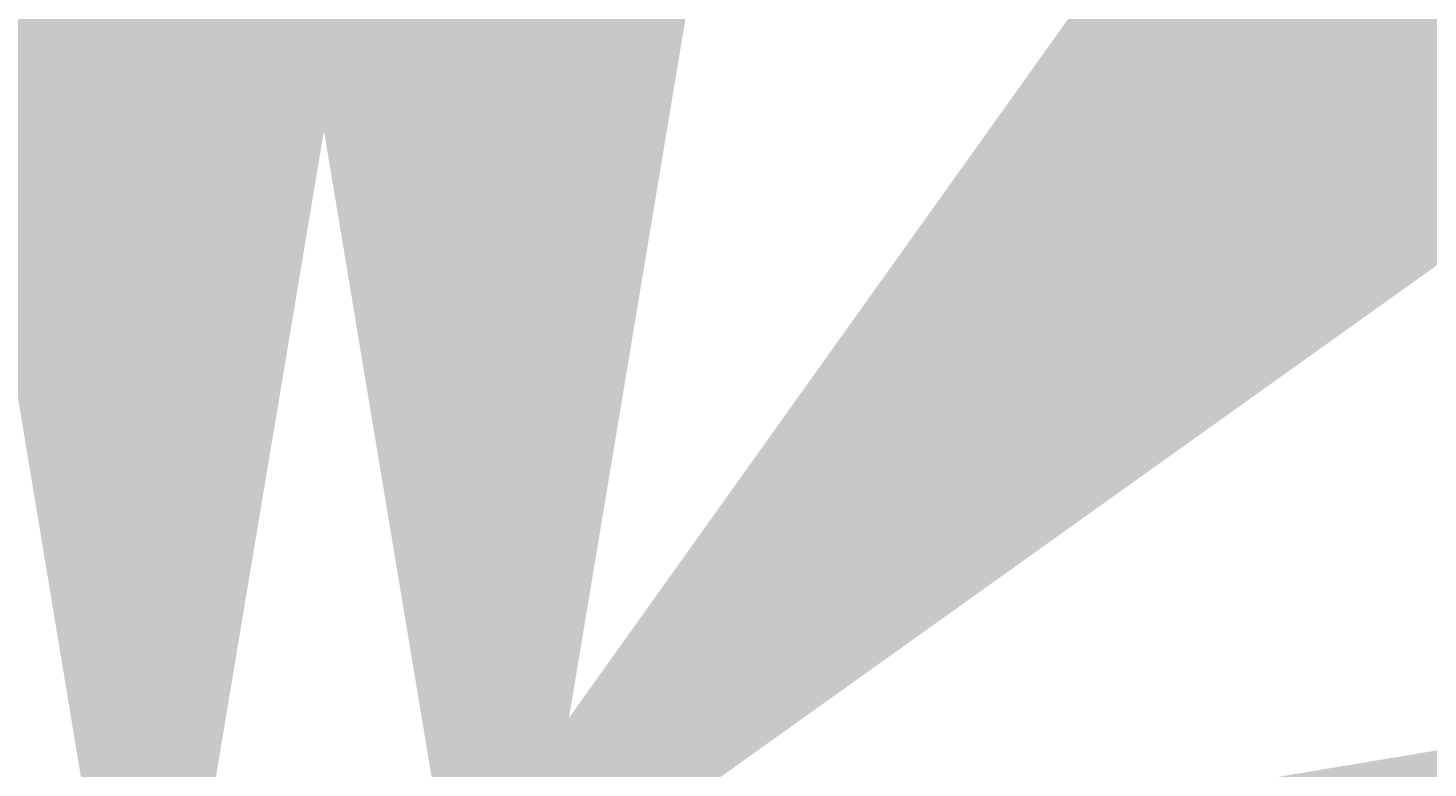
# Model space of a CAD drawing. Units: millimetres. Extents: x -22994 to 29398, y -19990 to 20176.
# Tile 128 of 135: x -44 to 1004, y 341 to 895. Entities that reach past the tile are written whole.
import ezdxf

# ---------------------------------------------------------------- set-up
doc = ezdxf.new("R2010")
doc.units = ezdxf.units.MM
doc.header["$MEASUREMENT"] = 0
doc.layers.add('M-DIMS', color=2, linetype='Continuous', lineweight=18)
doc.styles.get("Standard").update_dxf_attribs({"font": 'arial.ttf'})
doc.dimstyles.get("Standard").update_dxf_attribs({"dimtxt": 0.18, "dimasz": 10000, "dimexe": 0.18, "dimexo": 0.0625, "dimgap": 0.09, "dimtad": 0, "dimtih": 1, "dimtoh": 1, "dimdec": 0, "dimzin": 0, "dimdsep": 46, "dimtxsty": 'Standard', "dimcen": 0.09, "dimadec": 0, "dimazin": 0, "dimtfac": 1, "dimtdec": 0, "dimtofl": 0, "dimtmove": 0, "dimatfit": 3, "dimfxl": 1, "dimtolj": 1, "dimtzin": 0, "dimlwd": 30, "dimarcsym": 0})

# ---------------------------------------------------------------- blocks, each defined once
blk = doc.blocks.new('*D2')
at = {"layer": 'Defpoints', "color": 0, "transparency": 16777216}
for p in [(6.7, 10.3), (290.9, 10.3), (290.9, -5.1)]:
    blk.add_point(p, dxfattribs=at)
at = {"layer": 'M-DIMS', "color": 0, "lineweight": -2, "transparency": 16777216}
for p, q in [((6.7, 10.2), (6.7, -5.3)), ((290.9, 10.2), (290.9, -5.3))]:
    blk.add_line(p, q, dxfattribs=at)
at = {"layer": 'M-DIMS', "color": 0, "lineweight": 30, "transparency": 16777216}
for p, q in [((-9993.3, -5.1), (-19993.3, -5.1)), ((10290.9, -5.1), (20290.9, -5.1))]:
    blk.add_line(p, q, dxfattribs=at)
at = {"layer": 'M-DIMS', "color": 0, "transparency": 16777216}
for points in [[(-9993.3, 1661.6), (-9993.3, -1671.7), (6.7, -5.1)], [(10290.9, 1661.6), (10290.9, -1671.7), (290.9, -5.1)]]:
    blk.add_solid(points, dxfattribs=at)
at = {"layer": 'M-DIMS', "color": 0, "transparency": 16777216, "insert": (148.8, -5.1), "char_height": 0.18, "attachment_point": 5}
blk.add_mtext('\\A1;284.2', dxfattribs=at)
blk = doc.blocks.new('*D3')
at = {"layer": 'Defpoints', "color": 0, "transparency": 16777216}
for p in [(110.3, 204.2), (110.3, 176.4), (95.8, 128)]:
    blk.add_point(p, dxfattribs=at)
at = {"layer": 'M-DIMS', "color": 0, "lineweight": 30, "transparency": 16777216}
for p, q in [((-9904.2, 204.2), (-19904.2, 204.2)), ((10110.3, 204.2), (20110.3, 204.2))]:
    blk.add_line(p, q, dxfattribs=at)
at = {"layer": 'M-DIMS', "color": 0, "lineweight": -2, "transparency": 16777216}
for p, q in [((95.8, 128), (95.8, 204.3)), ((110.3, 176.4), (110.3, 204.3))]:
    blk.add_line(p, q, dxfattribs=at)
at = {"layer": 'M-DIMS', "color": 0, "transparency": 16777216}
for points in [[(-9904.2, 1870.8), (-9904.2, -1462.5), (95.8, 204.2)], [(10110.3, 1870.8), (10110.3, -1462.5), (110.3, 204.2)]]:
    blk.add_solid(points, dxfattribs=at)
at = {"layer": 'M-DIMS', "color": 0, "transparency": 16777216, "insert": (103, 204.2), "char_height": 0.18, "attachment_point": 5}
blk.add_mtext('\\A1;14.432', dxfattribs=at)
blk = doc.blocks.new('*D4')
at = {"layer": 'Defpoints', "color": 0, "transparency": 16777216}
for p in [(116.3, 204.2), (110.3, 176.4), (116.3, 176.4)]:
    blk.add_point(p, dxfattribs=at)
at = {"layer": 'M-DIMS', "color": 0, "lineweight": 30, "transparency": 16777216}
for p, q in [((-9889.7, 204.2), (-19889.7, 204.2)), ((10116.3, 204.2), (20116.3, 204.2))]:
    blk.add_line(p, q, dxfattribs=at)
at = {"layer": 'M-DIMS', "color": 0, "lineweight": -2, "transparency": 16777216}
for p, q in [((110.3, 176.4), (110.3, 204.3)), ((116.3, 176.4), (116.3, 204.3))]:
    blk.add_line(p, q, dxfattribs=at)
at = {"layer": 'M-DIMS', "color": 0, "transparency": 16777216}
for points in [[(-9889.7, 1870.8), (-9889.7, -1462.5), (110.3, 204.2)], [(10116.3, 1870.8), (10116.3, -1462.5), (116.3, 204.2)]]:
    blk.add_solid(points, dxfattribs=at)
at = {"layer": 'M-DIMS', "color": 0, "transparency": 16777216, "insert": (113.3, 204.2), "char_height": 0.18, "attachment_point": 5}
blk.add_mtext('\\A1;6', dxfattribs=at)
blk = doc.blocks.new('*D5')
at = {"layer": 'Defpoints', "color": 0, "transparency": 16777216}
for p in [(181.3, 204.2), (116.3, 176.4), (181.3, 176.4)]:
    blk.add_point(p, dxfattribs=at)
at = {"layer": 'M-DIMS', "color": 0, "lineweight": 30, "transparency": 16777216}
for p, q in [((-9883.7, 204.2), (-19883.7, 204.2)), ((10181.3, 204.2), (20181.3, 204.2))]:
    blk.add_line(p, q, dxfattribs=at)
at = {"layer": 'M-DIMS', "color": 0, "lineweight": -2, "transparency": 16777216}
for p, q in [((116.3, 176.4), (116.3, 204.3)), ((181.3, 176.4), (181.3, 204.3))]:
    blk.add_line(p, q, dxfattribs=at)
at = {"layer": 'M-DIMS', "color": 0, "transparency": 16777216}
for points in [[(-9883.7, 1870.8), (-9883.7, -1462.5), (116.3, 204.2)], [(10181.3, 1870.8), (10181.3, -1462.5), (181.3, 204.2)]]:
    blk.add_solid(points, dxfattribs=at)
at = {"layer": 'M-DIMS', "color": 0, "transparency": 16777216, "insert": (148.8, 204.2), "char_height": 0.18, "attachment_point": 5}
blk.add_mtext('\\A1;65', dxfattribs=at)
blk = doc.blocks.new('*D6')
at = {"layer": 'Defpoints', "color": 0, "transparency": 16777216}
for p in [(187.3, 204.2), (181.3, 176.4), (187.3, 176.4)]:
    blk.add_point(p, dxfattribs=at)
at = {"layer": 'M-DIMS', "color": 0, "lineweight": 30, "transparency": 16777216}
for p, q in [((-9818.7, 204.2), (-19818.7, 204.2)), ((10187.3, 204.2), (20187.3, 204.2))]:
    blk.add_line(p, q, dxfattribs=at)
at = {"layer": 'M-DIMS', "color": 0, "lineweight": -2, "transparency": 16777216}
for p, q in [((181.3, 176.4), (181.3, 204.3)), ((187.3, 176.4), (187.3, 204.3))]:
    blk.add_line(p, q, dxfattribs=at)
at = {"layer": 'M-DIMS', "color": 0, "transparency": 16777216}
for points in [[(-9818.7, 1870.8), (-9818.7, -1462.5), (181.3, 204.2)], [(10187.3, 1870.8), (10187.3, -1462.5), (187.3, 204.2)]]:
    blk.add_solid(points, dxfattribs=at)
at = {"layer": 'M-DIMS', "color": 0, "transparency": 16777216, "insert": (184.3, 204.2), "char_height": 0.18, "attachment_point": 5}
blk.add_mtext('\\A1;6', dxfattribs=at)
blk = doc.blocks.new('*D7')
at = {"layer": 'Defpoints', "color": 0, "transparency": 16777216}
for p in [(201.7, 204.2), (187.3, 176.4), (201.7, 128)]:
    blk.add_point(p, dxfattribs=at)
at = {"layer": 'M-DIMS', "color": 0, "lineweight": 30, "transparency": 16777216}
for p, q in [((-9812.7, 204.2), (-19812.7, 204.2)), ((10201.7, 204.2), (20201.7, 204.2))]:
    blk.add_line(p, q, dxfattribs=at)
at = {"layer": 'M-DIMS', "color": 0, "lineweight": -2, "transparency": 16777216}
for p, q in [((187.3, 176.4), (187.3, 204.3)), ((201.7, 128), (201.7, 204.3))]:
    blk.add_line(p, q, dxfattribs=at)
at = {"layer": 'M-DIMS', "color": 0, "transparency": 16777216}
for points in [[(-9812.7, 1870.8), (-9812.7, -1462.5), (187.3, 204.2)], [(10201.7, 1870.8), (10201.7, -1462.5), (201.7, 204.2)]]:
    blk.add_solid(points, dxfattribs=at)
at = {"layer": 'M-DIMS', "color": 0, "transparency": 16777216, "insert": (194.5, 204.2), "char_height": 0.18, "attachment_point": 5}
blk.add_mtext('\\A1;14.432', dxfattribs=at)
blk = doc.blocks.new('*D8')
at = {"layer": 'Defpoints', "color": 0, "transparency": 16777216}
for p in [(227.6, 204.2), (227.6, 146.7), (201.7, 128)]:
    blk.add_point(p, dxfattribs=at)
at = {"layer": 'M-DIMS', "color": 0, "lineweight": 30, "transparency": 16777216}
for p, q in [((-9798.3, 204.2), (-19798.3, 204.2)), ((10227.6, 204.2), (20227.6, 204.2))]:
    blk.add_line(p, q, dxfattribs=at)
at = {"layer": 'M-DIMS', "color": 0, "lineweight": -2, "transparency": 16777216}
for p, q in [((201.7, 128), (201.7, 204.3)), ((227.6, 146.8), (227.6, 204.3))]:
    blk.add_line(p, q, dxfattribs=at)
at = {"layer": 'M-DIMS', "color": 0, "transparency": 16777216}
for points in [[(-9798.3, 1870.8), (-9798.3, -1462.5), (201.7, 204.2)], [(10227.6, 1870.8), (10227.6, -1462.5), (227.6, 204.2)]]:
    blk.add_solid(points, dxfattribs=at)
at = {"layer": 'M-DIMS', "color": 0, "transparency": 16777216, "insert": (214.7, 204.2), "char_height": 0.18, "attachment_point": 5}
blk.add_mtext('\\A1;25.95', dxfattribs=at)
blk = doc.blocks.new('*D9')
at = {"layer": 'Defpoints', "color": 0, "transparency": 16777216}
for p in [(187.3, 176.4), (306.2, 176.4), (290.9, 10.3)]:
    blk.add_point(p, dxfattribs=at)
at = {"layer": 'M-DIMS', "color": 0, "lineweight": 30, "transparency": 16777216}
for p, q in [((306.2, 10176.4), (306.2, 20176.4)), ((306.2, -9989.7), (306.2, -19989.7))]:
    blk.add_line(p, q, dxfattribs=at)
at = {"layer": 'M-DIMS', "color": 0, "lineweight": -2, "transparency": 16777216}
for p, q in [((187.3, 176.4), (306.4, 176.4)), ((290.9, 10.3), (306.4, 10.3))]:
    blk.add_line(p, q, dxfattribs=at)
at = {"layer": 'M-DIMS', "color": 0, "transparency": 16777216}
for points in [[(-1360.5, 10176.4), (1972.9, 10176.4), (306.2, 176.4)], [(-1360.5, -9989.7), (1972.9, -9989.7), (306.2, 10.3)]]:
    blk.add_solid(points, dxfattribs=at)
at = {"layer": 'M-DIMS', "color": 0, "transparency": 16777216, "insert": (306.2, 93.3), "char_height": 0.18, "attachment_point": 5}
blk.add_mtext('\\A1;166.1', dxfattribs=at)
blk = doc.blocks.new('*D10')
at = {"layer": 'Defpoints', "color": 0, "transparency": 16777216}
for p in [(125.6, 136.1), (133.3, 136.1), (133.3, -5.1)]:
    blk.add_point(p, dxfattribs=at)
at = {"layer": 'M-DIMS', "color": 0, "lineweight": -2, "transparency": 16777216}
for p, q in [((125.6, 136), (125.6, -5.3)), ((133.3, 136), (133.3, -5.3))]:
    blk.add_line(p, q, dxfattribs=at)
at = {"layer": 'M-DIMS', "color": 0, "lineweight": 30, "transparency": 16777216}
for p, q in [((-9874.4, -5.1), (-19874.4, -5.1)), ((10133.3, -5.1), (20133.3, -5.1))]:
    blk.add_line(p, q, dxfattribs=at)
at = {"layer": 'M-DIMS', "color": 0, "transparency": 16777216}
for points in [[(-9874.4, 1661.6), (-9874.4, -1671.7), (125.6, -5.1)], [(10133.3, 1661.6), (10133.3, -1671.7), (133.3, -5.1)]]:
    blk.add_solid(points, dxfattribs=at)
at = {"layer": 'M-DIMS', "color": 0, "transparency": 16777216, "insert": (129.5, -5.1), "char_height": 0.18, "attachment_point": 5}
blk.add_mtext('\\A1;7.696', dxfattribs=at)
blk = doc.blocks.new('*D11')
at = {"layer": 'Defpoints', "color": 0, "transparency": 16777216}
for p in [(133.3, 136.1), (135.6, 136.1), (135.6, -5.1)]:
    blk.add_point(p, dxfattribs=at)
at = {"layer": 'M-DIMS', "color": 0, "lineweight": -2, "transparency": 16777216}
for p, q in [((133.3, 136), (133.3, -5.3)), ((135.6, 136), (135.6, -5.3))]:
    blk.add_line(p, q, dxfattribs=at)
at = {"layer": 'M-DIMS', "color": 0, "lineweight": 30, "transparency": 16777216}
for p, q in [((-9866.7, -5.1), (-19866.7, -5.1)), ((10135.6, -5.1), (20135.6, -5.1))]:
    blk.add_line(p, q, dxfattribs=at)
at = {"layer": 'M-DIMS', "color": 0, "transparency": 16777216}
for points in [[(-9866.7, 1661.6), (-9866.7, -1671.7), (133.3, -5.1)], [(10135.6, 1661.6), (10135.6, -1671.7), (135.6, -5.1)]]:
    blk.add_solid(points, dxfattribs=at)
at = {"layer": 'M-DIMS', "color": 0, "transparency": 16777216, "insert": (134.5, -5.1), "char_height": 0.18, "attachment_point": 5}
blk.add_mtext('\\A1;2.304', dxfattribs=at)
blk = doc.blocks.new('*D12')
at = {"layer": 'Defpoints', "color": 0, "transparency": 16777216}
for p in [(135.6, 136.1), (145.6, 136.1), (145.6, -5.1)]:
    blk.add_point(p, dxfattribs=at)
at = {"layer": 'M-DIMS', "color": 0, "lineweight": -2, "transparency": 16777216}
for p, q in [((135.6, 136), (135.6, -5.3)), ((145.6, 136), (145.6, -5.3))]:
    blk.add_line(p, q, dxfattribs=at)
at = {"layer": 'M-DIMS', "color": 0, "lineweight": 30, "transparency": 16777216}
for p, q in [((-9864.4, -5.1), (-19864.4, -5.1)), ((10145.6, -5.1), (20145.6, -5.1))]:
    blk.add_line(p, q, dxfattribs=at)
at = {"layer": 'M-DIMS', "color": 0, "transparency": 16777216}
for points in [[(-9864.4, 1661.6), (-9864.4, -1671.7), (135.6, -5.1)], [(10145.6, 1661.6), (10145.6, -1671.7), (145.6, -5.1)]]:
    blk.add_solid(points, dxfattribs=at)
at = {"layer": 'M-DIMS', "color": 0, "transparency": 16777216, "insert": (140.6, -5.1), "char_height": 0.18, "attachment_point": 5}
blk.add_mtext('\\A1;10', dxfattribs=at)
blk = doc.blocks.new('*D13')
at = {"layer": 'Defpoints', "color": 0, "transparency": 16777216}
for p in [(145.6, 136.1), (155.6, 136.1), (155.6, -5.1)]:
    blk.add_point(p, dxfattribs=at)
at = {"layer": 'M-DIMS', "color": 0, "lineweight": -2, "transparency": 16777216}
for p, q in [((145.6, 136), (145.6, -5.3)), ((155.6, 136), (155.6, -5.3))]:
    blk.add_line(p, q, dxfattribs=at)
at = {"layer": 'M-DIMS', "color": 0, "lineweight": 30, "transparency": 16777216}
for p, q in [((-9854.4, -5.1), (-19854.4, -5.1)), ((10155.6, -5.1), (20155.6, -5.1))]:
    blk.add_line(p, q, dxfattribs=at)
at = {"layer": 'M-DIMS', "color": 0, "transparency": 16777216}
for points in [[(-9854.4, 1661.6), (-9854.4, -1671.7), (145.6, -5.1)], [(10155.6, 1661.6), (10155.6, -1671.7), (155.6, -5.1)]]:
    blk.add_solid(points, dxfattribs=at)
at = {"layer": 'M-DIMS', "color": 0, "transparency": 16777216, "insert": (150.6, -5.1), "char_height": 0.18, "attachment_point": 5}
blk.add_mtext('\\A1;10', dxfattribs=at)
blk = doc.blocks.new('*D14')
at = {"layer": 'Defpoints', "color": 0, "transparency": 16777216}
for p in [(155.6, 136.1), (165.6, 136.1), (165.6, -5.1)]:
    blk.add_point(p, dxfattribs=at)
at = {"layer": 'M-DIMS', "color": 0, "lineweight": -2, "transparency": 16777216}
for p, q in [((155.6, 136), (155.6, -5.3)), ((165.6, 136), (165.6, -5.3))]:
    blk.add_line(p, q, dxfattribs=at)
at = {"layer": 'M-DIMS', "color": 0, "lineweight": 30, "transparency": 16777216}
for p, q in [((-9844.4, -5.1), (-19844.4, -5.1)), ((10165.6, -5.1), (20165.6, -5.1))]:
    blk.add_line(p, q, dxfattribs=at)
at = {"layer": 'M-DIMS', "color": 0, "transparency": 16777216}
for points in [[(-9844.4, 1661.6), (-9844.4, -1671.7), (155.6, -5.1)], [(10165.6, 1661.6), (10165.6, -1671.7), (165.6, -5.1)]]:
    blk.add_solid(points, dxfattribs=at)
at = {"layer": 'M-DIMS', "color": 0, "transparency": 16777216, "insert": (160.6, -5.1), "char_height": 0.18, "attachment_point": 5}
blk.add_mtext('\\A1;10', dxfattribs=at)
blk = doc.blocks.new('*D15')
at = {"layer": 'Defpoints', "color": 0, "transparency": 16777216}
for p in [(173.3, 154.8), (173.3, 136.1), (306.2, 136.1)]:
    blk.add_point(p, dxfattribs=at)
at = {"layer": 'M-DIMS', "color": 0, "lineweight": 30, "transparency": 16777216}
for p, q in [((306.2, 10154.8), (306.2, 20154.8)), ((306.2, -9863.9), (306.2, -19863.9))]:
    blk.add_line(p, q, dxfattribs=at)
at = {"layer": 'M-DIMS', "color": 0, "lineweight": -2, "transparency": 16777216}
for p, q in [((173.4, 154.8), (306.4, 154.8)), ((173.4, 136.1), (306.4, 136.1))]:
    blk.add_line(p, q, dxfattribs=at)
at = {"layer": 'M-DIMS', "color": 0, "transparency": 16777216}
for points in [[(-1360.5, 10154.8), (1972.9, 10154.8), (306.2, 154.8)], [(-1360.5, -9863.9), (1972.9, -9863.9), (306.2, 136.1)]]:
    blk.add_solid(points, dxfattribs=at)
at = {"layer": 'M-DIMS', "color": 0, "transparency": 16777216, "insert": (306.2, 145.4), "char_height": 0.18, "attachment_point": 5}
blk.add_mtext('\\A1;18.717', dxfattribs=at)
blk = doc.blocks.new('*D16')
at = {"layer": 'Defpoints', "color": 0, "transparency": 16777216}
for p in [(120.2, 204.2), (110.5, 48), (120.2, 48)]:
    blk.add_point(p, dxfattribs=at)
at = {"layer": 'M-DIMS', "color": 0, "lineweight": 30, "transparency": 16777216}
for p, q in [((-9889.5, 204.2), (-19889.5, 204.2)), ((10120.2, 204.2), (20120.2, 204.2))]:
    blk.add_line(p, q, dxfattribs=at)
at = {"layer": 'M-DIMS', "color": 0, "lineweight": -2, "transparency": 16777216}
for p, q in [((110.5, 48.1), (110.5, 204.3)), ((120.2, 48.1), (120.2, 204.3))]:
    blk.add_line(p, q, dxfattribs=at)
at = {"layer": 'M-DIMS', "color": 0, "transparency": 16777216}
for points in [[(-9889.5, 1870.8), (-9889.5, -1462.5), (110.5, 204.2)], [(10120.2, 1870.8), (10120.2, -1462.5), (120.2, 204.2)]]:
    blk.add_solid(points, dxfattribs=at)
at = {"layer": 'M-DIMS', "color": 0, "transparency": 16777216, "insert": (115.3, 204.2), "char_height": 0.18, "attachment_point": 5}
blk.add_mtext('\\A1;9.704', dxfattribs=at)
blk = doc.blocks.new('*D17')
at = {"layer": 'Defpoints', "color": 0, "transparency": 16777216}
for p in [(126.2, 204.2), (120.2, 48), (126.2, 48)]:
    blk.add_point(p, dxfattribs=at)
at = {"layer": 'M-DIMS', "color": 0, "lineweight": 30, "transparency": 16777216}
for p, q in [((-9879.8, 204.2), (-19879.8, 204.2)), ((10126.2, 204.2), (20126.2, 204.2))]:
    blk.add_line(p, q, dxfattribs=at)
at = {"layer": 'M-DIMS', "color": 0, "lineweight": -2, "transparency": 16777216}
for p, q in [((120.2, 48.1), (120.2, 204.3)), ((126.2, 48.1), (126.2, 204.3))]:
    blk.add_line(p, q, dxfattribs=at)
at = {"layer": 'M-DIMS', "color": 0, "transparency": 16777216}
for points in [[(-9879.8, 1870.8), (-9879.8, -1462.5), (120.2, 204.2)], [(10126.2, 1870.8), (10126.2, -1462.5), (126.2, 204.2)]]:
    blk.add_solid(points, dxfattribs=at)
at = {"layer": 'M-DIMS', "color": 0, "transparency": 16777216, "insert": (123.2, 204.2), "char_height": 0.18, "attachment_point": 5}
blk.add_mtext('\\A1;6', dxfattribs=at)
blk = doc.blocks.new('*D18')
at = {"layer": 'Defpoints', "color": 0, "transparency": 16777216}
for p in [(132.2, 204.2), (126.2, 48), (132.2, 48)]:
    blk.add_point(p, dxfattribs=at)
at = {"layer": 'M-DIMS', "color": 0, "lineweight": 30, "transparency": 16777216}
for p, q in [((-9873.8, 204.2), (-19873.8, 204.2)), ((10132.2, 204.2), (20132.2, 204.2))]:
    blk.add_line(p, q, dxfattribs=at)
at = {"layer": 'M-DIMS', "color": 0, "lineweight": -2, "transparency": 16777216}
for p, q in [((126.2, 48.1), (126.2, 204.3)), ((132.2, 48.1), (132.2, 204.3))]:
    blk.add_line(p, q, dxfattribs=at)
at = {"layer": 'M-DIMS', "color": 0, "transparency": 16777216}
for points in [[(-9873.8, 1870.8), (-9873.8, -1462.5), (126.2, 204.2)], [(10132.2, 1870.8), (10132.2, -1462.5), (132.2, 204.2)]]:
    blk.add_solid(points, dxfattribs=at)
at = {"layer": 'M-DIMS', "color": 0, "transparency": 16777216, "insert": (129.2, 204.2), "char_height": 0.18, "attachment_point": 5}
blk.add_mtext('\\A1;6', dxfattribs=at)
blk = doc.blocks.new('*D19')
at = {"layer": 'Defpoints', "color": 0, "transparency": 16777216}
for p in [(138.2, 204.2), (132.2, 48), (138.2, 48)]:
    blk.add_point(p, dxfattribs=at)
at = {"layer": 'M-DIMS', "color": 0, "lineweight": 30, "transparency": 16777216}
for p, q in [((-9867.8, 204.2), (-19867.8, 204.2)), ((10138.2, 204.2), (20138.2, 204.2))]:
    blk.add_line(p, q, dxfattribs=at)
at = {"layer": 'M-DIMS', "color": 0, "lineweight": -2, "transparency": 16777216}
for p, q in [((132.2, 48.1), (132.2, 204.3)), ((138.2, 48.1), (138.2, 204.3))]:
    blk.add_line(p, q, dxfattribs=at)
at = {"layer": 'M-DIMS', "color": 0, "transparency": 16777216}
for points in [[(-9867.8, 1870.8), (-9867.8, -1462.5), (132.2, 204.2)], [(10138.2, 1870.8), (10138.2, -1462.5), (138.2, 204.2)]]:
    blk.add_solid(points, dxfattribs=at)
at = {"layer": 'M-DIMS', "color": 0, "transparency": 16777216, "insert": (135.2, 204.2), "char_height": 0.18, "attachment_point": 5}
blk.add_mtext('\\A1;6', dxfattribs=at)
blk = doc.blocks.new('*D20')
at = {"layer": 'Defpoints', "color": 0, "transparency": 16777216}
for p in [(144.2, 204.2), (138.2, 48), (144.2, 48)]:
    blk.add_point(p, dxfattribs=at)
at = {"layer": 'M-DIMS', "color": 0, "lineweight": 30, "transparency": 16777216}
for p, q in [((-9861.8, 204.2), (-19861.8, 204.2)), ((10144.2, 204.2), (20144.2, 204.2))]:
    blk.add_line(p, q, dxfattribs=at)
at = {"layer": 'M-DIMS', "color": 0, "lineweight": -2, "transparency": 16777216}
for p, q in [((138.2, 48.1), (138.2, 204.3)), ((144.2, 48.1), (144.2, 204.3))]:
    blk.add_line(p, q, dxfattribs=at)
at = {"layer": 'M-DIMS', "color": 0, "transparency": 16777216}
for points in [[(-9861.8, 1870.8), (-9861.8, -1462.5), (138.2, 204.2)], [(10144.2, 1870.8), (10144.2, -1462.5), (144.2, 204.2)]]:
    blk.add_solid(points, dxfattribs=at)
at = {"layer": 'M-DIMS', "color": 0, "transparency": 16777216, "insert": (141.2, 204.2), "char_height": 0.18, "attachment_point": 5}
blk.add_mtext('\\A1;6', dxfattribs=at)
blk = doc.blocks.new('*D21')
at = {"layer": 'Defpoints', "color": 0, "transparency": 16777216}
for p in [(149.1, 204.2), (144.2, 48), (149.1, 48)]:
    blk.add_point(p, dxfattribs=at)
at = {"layer": 'M-DIMS', "color": 0, "lineweight": 30, "transparency": 16777216}
for p, q in [((-9855.8, 204.2), (-19855.8, 204.2)), ((10149.1, 204.2), (20149.1, 204.2))]:
    blk.add_line(p, q, dxfattribs=at)
at = {"layer": 'M-DIMS', "color": 0, "lineweight": -2, "transparency": 16777216}
for p, q in [((144.2, 48.1), (144.2, 204.3)), ((149.1, 48.1), (149.1, 204.3))]:
    blk.add_line(p, q, dxfattribs=at)
at = {"layer": 'M-DIMS', "color": 0, "transparency": 16777216}
for points in [[(-9855.8, 1870.8), (-9855.8, -1462.5), (144.2, 204.2)], [(10149.1, 1870.8), (10149.1, -1462.5), (149.1, 204.2)]]:
    blk.add_solid(points, dxfattribs=at)
at = {"layer": 'M-DIMS', "color": 0, "transparency": 16777216, "insert": (146.6, 204.2), "char_height": 0.18, "attachment_point": 5}
blk.add_mtext('\\A1;4.945', dxfattribs=at)
blk = doc.blocks.new('*D22')
at = {"layer": 'Defpoints', "color": 0, "transparency": 16777216}
for p in [(149.1, 31), (155.1, 31), (155.1, -5.1)]:
    blk.add_point(p, dxfattribs=at)
at = {"layer": 'M-DIMS', "color": 0, "lineweight": -2, "transparency": 16777216}
for p, q in [((149.1, 30.9), (149.1, -5.3)), ((155.1, 30.9), (155.1, -5.3))]:
    blk.add_line(p, q, dxfattribs=at)
at = {"layer": 'M-DIMS', "color": 0, "lineweight": 30, "transparency": 16777216}
for p, q in [((-9850.9, -5.1), (-19850.9, -5.1)), ((10155.1, -5.1), (20155.1, -5.1))]:
    blk.add_line(p, q, dxfattribs=at)
at = {"layer": 'M-DIMS', "color": 0, "transparency": 16777216}
for points in [[(-9850.9, 1661.6), (-9850.9, -1671.7), (149.1, -5.1)], [(10155.1, 1661.6), (10155.1, -1671.7), (155.1, -5.1)]]:
    blk.add_solid(points, dxfattribs=at)
at = {"layer": 'M-DIMS', "color": 0, "transparency": 16777216, "insert": (152.1, -5.1), "char_height": 0.18, "attachment_point": 5}
blk.add_mtext('\\A1;6', dxfattribs=at)
blk = doc.blocks.new('*D23')
at = {"layer": 'Defpoints', "color": 0, "transparency": 16777216}
for p in [(155.1, 31), (161.1, 31), (161.1, -5.1)]:
    blk.add_point(p, dxfattribs=at)
at = {"layer": 'M-DIMS', "color": 0, "lineweight": -2, "transparency": 16777216}
for p, q in [((155.1, 30.9), (155.1, -5.3)), ((161.1, 30.9), (161.1, -5.3))]:
    blk.add_line(p, q, dxfattribs=at)
at = {"layer": 'M-DIMS', "color": 0, "lineweight": 30, "transparency": 16777216}
for p, q in [((-9844.9, -5.1), (-19844.9, -5.1)), ((10161.1, -5.1), (20161.1, -5.1))]:
    blk.add_line(p, q, dxfattribs=at)
at = {"layer": 'M-DIMS', "color": 0, "transparency": 16777216}
for points in [[(-9844.9, 1661.6), (-9844.9, -1671.7), (155.1, -5.1)], [(10161.1, 1661.6), (10161.1, -1671.7), (161.1, -5.1)]]:
    blk.add_solid(points, dxfattribs=at)
at = {"layer": 'M-DIMS', "color": 0, "transparency": 16777216, "insert": (158.1, -5.1), "char_height": 0.18, "attachment_point": 5}
blk.add_mtext('\\A1;6', dxfattribs=at)
blk = doc.blocks.new('*D24')
at = {"layer": 'Defpoints', "color": 0, "transparency": 16777216}
for p in [(161.1, 31), (166.4, 31), (166.4, -5.1)]:
    blk.add_point(p, dxfattribs=at)
at = {"layer": 'M-DIMS', "color": 0, "lineweight": -2, "transparency": 16777216}
for p, q in [((161.1, 30.9), (161.1, -5.3)), ((166.4, 30.9), (166.4, -5.3))]:
    blk.add_line(p, q, dxfattribs=at)
at = {"layer": 'M-DIMS', "color": 0, "lineweight": 30, "transparency": 16777216}
for p, q in [((-9838.9, -5.1), (-19838.9, -5.1)), ((10166.4, -5.1), (20166.4, -5.1))]:
    blk.add_line(p, q, dxfattribs=at)
at = {"layer": 'M-DIMS', "color": 0, "transparency": 16777216}
for points in [[(-9838.9, 1661.6), (-9838.9, -1671.7), (161.1, -5.1)], [(10166.4, 1661.6), (10166.4, -1671.7), (166.4, -5.1)]]:
    blk.add_solid(points, dxfattribs=at)
at = {"layer": 'M-DIMS', "color": 0, "transparency": 16777216, "insert": (163.8, -5.1), "char_height": 0.18, "attachment_point": 5}
blk.add_mtext('\\A1;5.323', dxfattribs=at)
blk = doc.blocks.new('*D25')
at = {"layer": 'Defpoints', "color": 0, "transparency": 16777216}
for p in [(166.4, 31), (172.4, 31), (172.4, -5.1)]:
    blk.add_point(p, dxfattribs=at)
at = {"layer": 'M-DIMS', "color": 0, "lineweight": -2, "transparency": 16777216}
for p, q in [((166.4, 30.9), (166.4, -5.3)), ((172.4, 30.9), (172.4, -5.3))]:
    blk.add_line(p, q, dxfattribs=at)
at = {"layer": 'M-DIMS', "color": 0, "lineweight": 30, "transparency": 16777216}
for p, q in [((-9833.6, -5.1), (-19833.6, -5.1)), ((10172.4, -5.1), (20172.4, -5.1))]:
    blk.add_line(p, q, dxfattribs=at)
at = {"layer": 'M-DIMS', "color": 0, "transparency": 16777216}
for points in [[(-9833.6, 1661.6), (-9833.6, -1671.7), (166.4, -5.1)], [(10172.4, 1661.6), (10172.4, -1671.7), (172.4, -5.1)]]:
    blk.add_solid(points, dxfattribs=at)
at = {"layer": 'M-DIMS', "color": 0, "transparency": 16777216, "insert": (169.4, -5.1), "char_height": 0.18, "attachment_point": 5}
blk.add_mtext('\\A1;6', dxfattribs=at)
blk = doc.blocks.new('*D26')
at = {"layer": 'Defpoints', "color": 0, "transparency": 16777216}
for p in [(172.4, 31), (178.4, 31), (178.4, -5.1)]:
    blk.add_point(p, dxfattribs=at)
at = {"layer": 'M-DIMS', "color": 0, "lineweight": -2, "transparency": 16777216}
for p, q in [((172.4, 30.9), (172.4, -5.3)), ((178.4, 30.9), (178.4, -5.3))]:
    blk.add_line(p, q, dxfattribs=at)
at = {"layer": 'M-DIMS', "color": 0, "lineweight": 30, "transparency": 16777216}
for p, q in [((-9827.6, -5.1), (-19827.6, -5.1)), ((10178.4, -5.1), (20178.4, -5.1))]:
    blk.add_line(p, q, dxfattribs=at)
at = {"layer": 'M-DIMS', "color": 0, "transparency": 16777216}
for points in [[(-9827.6, 1661.6), (-9827.6, -1671.7), (172.4, -5.1)], [(10178.4, 1661.6), (10178.4, -1671.7), (178.4, -5.1)]]:
    blk.add_solid(points, dxfattribs=at)
at = {"layer": 'M-DIMS', "color": 0, "transparency": 16777216, "insert": (175.4, -5.1), "char_height": 0.18, "attachment_point": 5}
blk.add_mtext('\\A1;6', dxfattribs=at)
blk = doc.blocks.new('*D27')
at = {"layer": 'Defpoints', "color": 0, "transparency": 16777216}
for p in [(178.4, 31), (188.1, 31), (188.1, -5.1)]:
    blk.add_point(p, dxfattribs=at)
at = {"layer": 'M-DIMS', "color": 0, "lineweight": -2, "transparency": 16777216}
for p, q in [((178.4, 30.9), (178.4, -5.3)), ((188.1, 30.9), (188.1, -5.3))]:
    blk.add_line(p, q, dxfattribs=at)
at = {"layer": 'M-DIMS', "color": 0, "lineweight": 30, "transparency": 16777216}
for p, q in [((-9821.6, -5.1), (-19821.6, -5.1)), ((10188.1, -5.1), (20188.1, -5.1))]:
    blk.add_line(p, q, dxfattribs=at)
at = {"layer": 'M-DIMS', "color": 0, "transparency": 16777216}
for points in [[(-9821.6, 1661.6), (-9821.6, -1671.7), (178.4, -5.1)], [(10188.1, 1661.6), (10188.1, -1671.7), (188.1, -5.1)]]:
    blk.add_solid(points, dxfattribs=at)
at = {"layer": 'M-DIMS', "color": 0, "transparency": 16777216, "insert": (183.3, -5.1), "char_height": 0.18, "attachment_point": 5}
blk.add_mtext('\\A1;9.679', dxfattribs=at)
blk = doc.blocks.new('*D28')
at = {"layer": 'Defpoints', "color": 0, "transparency": 16777216}
for p in [(188.1, 48), (306.2, 48), (188.1, 31)]:
    blk.add_point(p, dxfattribs=at)
at = {"layer": 'M-DIMS', "color": 0, "lineweight": 30, "transparency": 16777216}
for p, q in [((306.2, 10048), (306.2, 20048)), ((306.2, -9969), (306.2, -19969))]:
    blk.add_line(p, q, dxfattribs=at)
at = {"layer": 'M-DIMS', "color": 0, "lineweight": -2, "transparency": 16777216}
for p, q in [((188.2, 48), (306.4, 48)), ((188.2, 31), (306.4, 31))]:
    blk.add_line(p, q, dxfattribs=at)
at = {"layer": 'M-DIMS', "color": 0, "transparency": 16777216}
for points in [[(-1360.5, 10048), (1972.9, 10048), (306.2, 48)], [(-1360.5, -9969), (1972.9, -9969), (306.2, 31)]]:
    blk.add_solid(points, dxfattribs=at)
at = {"layer": 'M-DIMS', "color": 0, "transparency": 16777216, "insert": (306.2, 39.5), "char_height": 0.18, "attachment_point": 5}
blk.add_mtext('\\A1;17.045', dxfattribs=at)
blk = doc.blocks.new('*D29')
at = {"layer": 'Defpoints', "color": 0, "transparency": 16777216}
for p in [(36.8, 80), (64, 80)]:
    blk.add_point(p, dxfattribs=at)
at = {"layer": 'M-DIMS', "color": 0, "lineweight": -2, "transparency": 16777216}
for p, q in [((50.3, 80), (50.5, 80)), ((50.4, 80), (50.4, 80.1))]:
    blk.add_line(p, q, dxfattribs=at)
at = {"layer": 'M-DIMS', "color": 0, "lineweight": 30, "transparency": 16777216}
blk.add_line((20064, 80), (10064, 80), dxfattribs=at)
at = {"layer": 'M-DIMS', "color": 0, "transparency": 16777216}
blk.add_solid([(10064, 1746.7), (10064, -1586.6), (64, 80)], dxfattribs=at)
at = {"layer": 'M-DIMS', "color": 0, "transparency": 16777216, "insert": (20064.5, 80), "char_height": 0.18, "attachment_point": 5}
blk.add_mtext('\\A1;∅27.23', dxfattribs=at)
blk = doc.blocks.new('*D30')
at = {"layer": 'Defpoints', "color": 0, "transparency": 16777216}
for p in [(216.3, 146.7), (239, 146.7)]:
    blk.add_point(p, dxfattribs=at)
at = {"layer": 'M-DIMS', "color": 0, "lineweight": -2, "transparency": 16777216}
for p, q in [((227.6, 146.6), (227.6, 146.8)), ((227.6, 146.7), (227.7, 146.7))]:
    blk.add_line(p, q, dxfattribs=at)
at = {"layer": 'M-DIMS', "color": 0, "lineweight": 30, "transparency": 16777216}
blk.add_line((20239, 147.5), (10239, 147.1), dxfattribs=at)
at = {"layer": 'M-DIMS', "color": 0, "transparency": 16777216}
blk.add_solid([(10238.9, 1813.8), (10239, -1519.6), (239, 146.7)], dxfattribs=at)
at = {"layer": 'M-DIMS', "color": 0, "transparency": 16777216, "insert": (20239.5, 147.5), "char_height": 0.18, "attachment_point": 5}
blk.add_mtext('\\A1;∅22.667', dxfattribs=at)
blk = doc.blocks.new('*D31')
at = {"layer": 'Defpoints', "color": 0, "transparency": 16777216}
for p in [(223.2, 146.7), (232.1, 146.7)]:
    blk.add_point(p, dxfattribs=at)
at = {"layer": 'M-DIMS', "color": 0, "lineweight": -2, "transparency": 16777216}
for p, q in [((227.6, 146.6), (227.6, 146.8)), ((227.6, 146.7), (227.7, 146.7))]:
    blk.add_line(p, q, dxfattribs=at)
at = {"layer": 'M-DIMS', "color": 0, "lineweight": 30, "transparency": 16777216}
blk.add_line((20232.1, 148.7), (10232.1, 147.7), dxfattribs=at)
at = {"layer": 'M-DIMS', "color": 0, "transparency": 16777216}
blk.add_solid([(10232, 1814.4), (10232.3, -1519), (232.1, 146.7)], dxfattribs=at)
at = {"layer": 'M-DIMS', "color": 0, "transparency": 16777216, "insert": (20232.6, 148.7), "char_height": 0.18, "attachment_point": 5}
blk.add_mtext('\\A1;∅8.969', dxfattribs=at)
blk = doc.blocks.new('*D34')
at = {"layer": 'Defpoints', "color": 0, "transparency": 16777216}
for p in [(176.8, 121.1), (178.6, 122.9)]:
    blk.add_point(p, dxfattribs=at)
at = {"layer": 'M-DIMS', "color": 0, "lineweight": 30, "transparency": 16777216}
for p, q in [((14322.4, 14263.3), (7250.5, 7193.1)), ((24322.4, 14263.3), (14322.4, 14263.3))]:
    blk.add_line(p, q, dxfattribs=at)
at = {"layer": 'M-DIMS', "color": 0, "lineweight": -2, "transparency": 16777216}
for p, q in [((176.7, 121.1), (176.9, 121.1)), ((176.8, 121), (176.8, 121.2))]:
    blk.add_line(p, q, dxfattribs=at)
at = {"layer": 'M-DIMS', "color": 0, "transparency": 16777216}
blk.add_solid([(6072.1, 8371.8), (8428.9, 6014.4), (178.6, 122.9)], dxfattribs=at)
at = {"layer": 'M-DIMS', "color": 0, "transparency": 16777216, "insert": (24323, 14263.3), "char_height": 0.18, "attachment_point": 5}
blk.add_mtext('\\A1;6X R2.5', dxfattribs=at)
blk = doc.blocks.new('*D35')
at = {"layer": 'Defpoints', "color": 0, "transparency": 16777216}
for p in [(21.1, 77.4), (21.8, 76.1)]:
    blk.add_point(p, dxfattribs=at)
at = {"layer": 'M-DIMS', "color": 0, "lineweight": 30, "transparency": 16777216}
for p, q in [((-19938, 17421.4), (-9938, 17421.4)), ((-9938, 17421.4), (-4958.5, 8749.4))]:
    blk.add_line(p, q, dxfattribs=at)
at = {"layer": 'M-DIMS', "color": 0, "lineweight": -2, "transparency": 16777216}
for p, q in [((21.8, 76), (21.8, 76.2)), ((21.8, 76.1), (21.9, 76.1))]:
    blk.add_line(p, q, dxfattribs=at)
at = {"layer": 'M-DIMS', "color": 0, "transparency": 16777216}
blk.add_solid([(-3513.1, 9579.3), (-6403.8, 7919.5), (21.1, 77.4)], dxfattribs=at)
at = {"layer": 'M-DIMS', "color": 0, "transparency": 16777216, "insert": (-19938.4, 17421.4), "char_height": 0.18, "attachment_point": 5}
blk.add_mtext('\\A1;R1.5', dxfattribs=at)
blk = doc.blocks.new('*D36')
at = {"layer": 'Defpoints', "color": 0, "transparency": 16777216}
for p in [(46.4, 31.3), (46.4, 26.6)]:
    blk.add_point(p, dxfattribs=at)
at = {"layer": 'M-DIMS', "color": 0, "lineweight": 30, "transparency": 16777216}
for p, q in [((57.1, 20031.3), (51.8, 10031.3)), ((10057.1, 20031.3), (57.1, 20031.3))]:
    blk.add_line(p, q, dxfattribs=at)
at = {"layer": 'M-DIMS', "color": 0, "lineweight": -2, "transparency": 16777216}
for p, q in [((46.3, 28.9), (46.5, 28.9)), ((46.4, 28.9), (46.4, 29))]:
    blk.add_line(p, q, dxfattribs=at)
at = {"layer": 'M-DIMS', "color": 0, "transparency": 16777216}
blk.add_solid([(-1614.9, 10032.2), (1718.4, 10030.4), (46.4, 31.3)], dxfattribs=at)
at = {"layer": 'M-DIMS', "color": 0, "transparency": 16777216, "insert": (10057.6, 20031.3), "char_height": 0.18, "attachment_point": 5}
blk.add_mtext('\\A1;∅4.71', dxfattribs=at)
blk = doc.blocks.new('*D37')
at = {"layer": 'Defpoints', "color": 0, "transparency": 16777216}
for p in [(54.8, 118.6), (59.5, 118.6)]:
    blk.add_point(p, dxfattribs=at)
at = {"layer": 'M-DIMS', "color": 0, "lineweight": -2, "transparency": 16777216}
for p, q in [((57.1, 118.6), (57.3, 118.6)), ((57.2, 118.5), (57.2, 118.7))]:
    blk.add_line(p, q, dxfattribs=at)
at = {"layer": 'M-DIMS', "color": 0, "lineweight": 30, "transparency": 16777216}
blk.add_line((20059.5, 116.3), (10059.5, 117.4), dxfattribs=at)
at = {"layer": 'M-DIMS', "color": 0, "transparency": 16777216}
blk.add_solid([(10059.7, 1784.1), (10059.3, -1549.2), (59.5, 118.6)], dxfattribs=at)
at = {"layer": 'M-DIMS', "color": 0, "transparency": 16777216, "insert": (20060, 116.3), "char_height": 0.18, "attachment_point": 5}
blk.add_mtext('\\A1;∅4.659', dxfattribs=at)

msp = doc.modelspace()

# ---------------------------------------------------------------- dimensions: what is measured, and where the dimension line sits
at = {"layer": 'M-DIMS'}
for base, p1, p2, override, picture, middle in [((306.202, 176.3662), (290.852, 10.2713), (187.2647, 176.3662), {"dimdec": 1, "dimlfac": 1, "dimrnd": 0, "dimzin": 0, "dimdsep": 46, "dimlunit": 2}, '*D9', (306.202, 93.3187)), ((306.202, 136.0713), (173.3459, 154.788), (173.3459, 136.0713), {"dimdec": 3, "dimlfac": 1, "dimrnd": 0, "dimzin": 0, "dimdsep": 46, "dimlunit": 2}, '*D15', (306.202, 145.4297)), ((306.202, 48.0349), (188.1175, 30.9895), (188.1175, 48.0349), {"dimdec": 3, "dimlfac": 1, "dimrnd": 0, "dimzin": 0, "dimdsep": 46, "dimlunit": 2}, '*D28', (306.202, 39.5122))]:
    dim = msp.add_linear_dim(base=base, p1=p1, p2=p2, angle=90, dimstyle='Standard', override=override, dxfattribs=at)
    dim.commit()
    dim.dimension.update_dxf_attribs({"geometry": picture, "text_midpoint": middle})
for p1, p2, override, picture, middle in [((46.3875, 26.5934), (46.39, 31.3035), {"dimdec": 2, "dimlfac": 1, "dimrnd": 0, "dimzin": 0, "dimdsep": 46, "dimlunit": 2}, '*D36', (10057.5542, 20031.3006)), ((216.3148, 146.7291), (238.9821, 146.73), {"dimdec": 3, "dimlfac": 1, "dimrnd": 0, "dimzin": 0, "dimdsep": 46, "dimlunit": 2}, '*D30', (20238.9821, 147.4959)), ((223.1641, 146.7291), (232.1328, 146.73), {"dimdec": 3, "dimlfac": 1, "dimrnd": 0, "dimzin": 0, "dimdsep": 46, "dimlunit": 2}, '*D31', (20232.1327, 148.6656))]:
    dim = msp.add_diameter_dim_2p(p1=p1, p2=p2, dimstyle='Standard', override=override, dxfattribs=at)
    dim.commit()
    dim.dimension.update_dxf_attribs({"geometry": picture, "text_midpoint": middle, "dimtype": 163})
dim = msp.add_radius_dim(center=(21.8402, 76.0922), mpoint=(21.0933, 77.393), dimstyle='Standard', override={"dimdec": 1, "dimlfac": 1, "dimrnd": 0, "dimzin": 0, "dimdsep": 46, "dimlunit": 2}, dxfattribs=at)
dim.commit()
dim.dimension.update_dxf_attribs({"geometry": '*D35', "text_midpoint": (-19938.3541, 17421.4466)})
dim = msp.add_radius_dim(center=(176.8123, 121.1277), mpoint=(178.5802, 122.8952), text='6X <>', dimstyle='Standard', override={"dimdec": 1, "dimlfac": 1, "dimrnd": 0, "dimzin": 0, "dimdsep": 46, "dimlunit": 2}, dxfattribs=at)
dim.commit()
dim.dimension.update_dxf_attribs({"geometry": '*D34', "text_midpoint": (24322.9703, 14263.3108)})
for base, p1, p2, override, picture, middle in [((110.2647, 204.1654), (95.8327, 127.967), (110.2647, 176.3662), {"dimdec": 3, "dimlfac": 1, "dimrnd": 0, "dimzin": 0, "dimdsep": 46, "dimlunit": 2}, '*D3', (103.0487, 204.1654)), ((116.2647, 204.1654), (110.2647, 176.3662), (116.2647, 176.3662), {"dimdec": 0, "dimlfac": 1, "dimrnd": 0, "dimzin": 0, "dimdsep": 46, "dimlunit": 2}, '*D4', (113.2647, 204.1654)), ((120.1702, 204.1654), (110.4658, 48.0349), (120.1702, 48.0349), {"dimdec": 3, "dimlfac": 1, "dimrnd": 0, "dimzin": 0, "dimdsep": 46, "dimlunit": 2}, '*D16', (115.318, 204.1654)), ((181.2647, 204.1654), (116.2647, 176.3662), (181.2647, 176.3662), {"dimdec": 0, "dimlfac": 1, "dimrnd": 0, "dimzin": 0, "dimdsep": 46, "dimlunit": 2}, '*D5', (148.7647, 204.1654)), ((126.1702, 204.1654), (120.1702, 48.0349), (126.1702, 48.0349), {"dimdec": 0, "dimlfac": 1, "dimrnd": 0, "dimzin": 0, "dimdsep": 46, "dimlunit": 2}, '*D17', (123.1702, 204.1654)), ((132.1702, 204.1654), (126.1702, 48.0349), (132.1702, 48.0349), {"dimdec": 0, "dimlfac": 1, "dimrnd": 0, "dimzin": 0, "dimdsep": 46, "dimlunit": 2}, '*D18', (129.1702, 204.1654)), ((138.1702, 204.1654), (132.1702, 48.0349), (138.1702, 48.0349), {"dimdec": 0, "dimlfac": 1, "dimrnd": 0, "dimzin": 0, "dimdsep": 46, "dimlunit": 2}, '*D19', (135.1702, 204.1654)), ((144.1702, 204.1654), (138.1702, 48.0349), (144.1702, 48.0349), {"dimdec": 0, "dimlfac": 1, "dimrnd": 0, "dimzin": 0, "dimdsep": 46, "dimlunit": 2}, '*D20', (141.1702, 204.1654)), ((149.11567, 204.16539), (144.17023, 48.03494), (149.11567, 48.03494), {"dimdec": 3, "dimlfac": 1, "dimrnd": 0, "dimzin": 0, "dimdsep": 46, "dimlunit": 2}, '*D21', (146.64295, 204.16539)), ((187.2647, 204.1654), (181.2647, 176.3662), (187.2647, 176.3662), {"dimdec": 0, "dimlfac": 1, "dimrnd": 0, "dimzin": 0, "dimdsep": 46, "dimlunit": 2}, '*D6', (184.2647, 204.1654)), ((201.6967, 204.1654), (187.2647, 176.3662), (201.6967, 127.967), {"dimdec": 3, "dimlfac": 1, "dimrnd": 0, "dimzin": 0, "dimdsep": 46, "dimlunit": 2}, '*D7', (194.4807, 204.1654)), ((227.6485, 204.1654), (201.6967, 127.967), (227.6485, 146.7296), {"dimdec": 2, "dimlfac": 1, "dimrnd": 0, "dimzin": 0, "dimdsep": 46, "dimlunit": 2}, '*D8', (214.6726, 204.1654)), ((290.852, -5.0787), (6.6773, 10.2713), (290.852, 10.2713), {"dimdec": 1, "dimlfac": 1, "dimrnd": 0, "dimzin": 0, "dimdsep": 46, "dimlunit": 2}, '*D2', (148.7647, -5.0787)), ((133.3459, -5.0787), (125.6498, 136.0713), (133.3459, 136.0713), {"dimdec": 3, "dimlfac": 1, "dimrnd": 0, "dimzin": 0, "dimdsep": 46, "dimlunit": 2}, '*D10', (129.4978, -5.0787)), ((135.6498, -5.0787), (133.3459, 136.0713), (135.6498, 136.0713), {"dimdec": 3, "dimlfac": 1, "dimrnd": 0, "dimzin": 0, "dimdsep": 46, "dimlunit": 2}, '*D11', (134.4978, -5.0787)), ((145.6498, -5.0787), (135.6498, 136.0713), (145.6498, 136.0713), {"dimdec": 0, "dimlfac": 1, "dimrnd": 0, "dimzin": 0, "dimdsep": 46, "dimlunit": 2}, '*D12', (140.6498, -5.0787)), ((155.6498, -5.0787), (145.6498, 136.0713), (155.6498, 136.0713), {"dimdec": 0, "dimlfac": 1, "dimrnd": 0, "dimzin": 0, "dimdsep": 46, "dimlunit": 2}, '*D13', (150.6498, -5.0787)), ((155.1157, -5.0787), (149.1157, 30.9895), (155.1157, 30.9895), {"dimdec": 0, "dimlfac": 1, "dimrnd": 0, "dimzin": 0, "dimdsep": 46, "dimlunit": 2}, '*D22', (152.1157, -5.0787)), ((161.1157, -5.0787), (155.1157, 30.9895), (161.1157, 30.9895), {"dimdec": 0, "dimlfac": 1, "dimrnd": 0, "dimzin": 0, "dimdsep": 46, "dimlunit": 2}, '*D23', (158.1157, -5.0787)), ((165.6498, -5.0787), (155.6498, 136.0713), (165.6498, 136.0713), {"dimdec": 0, "dimlfac": 1, "dimrnd": 0, "dimzin": 0, "dimdsep": 46, "dimlunit": 2}, '*D14', (160.6498, -5.0787)), ((166.4387, -5.0787), (161.1157, 30.9895), (166.4387, 30.9895), {"dimdec": 3, "dimlfac": 1, "dimrnd": 0, "dimzin": 0, "dimdsep": 46, "dimlunit": 2}, '*D24', (163.7772, -5.0787)), ((172.4387, -5.0787), (166.4387, 30.9895), (172.4387, 30.9895), {"dimdec": 0, "dimlfac": 1, "dimrnd": 0, "dimzin": 0, "dimdsep": 46, "dimlunit": 2}, '*D25', (169.4387, -5.0787)), ((178.4387, -5.0787), (172.4387, 30.9895), (178.4387, 30.9895), {"dimdec": 0, "dimlfac": 1, "dimrnd": 0, "dimzin": 0, "dimdsep": 46, "dimlunit": 2}, '*D26', (175.4387, -5.0787)), ((188.1175, -5.0787), (178.4387, 30.9895), (188.1175, 30.9895), {"dimdec": 3, "dimlfac": 1, "dimrnd": 0, "dimzin": 0, "dimdsep": 46, "dimlunit": 2}, '*D27', (183.2781, -5.0787))]:
    dim = msp.add_linear_dim(base=base, p1=p1, p2=p2, dimstyle='Standard', override=override, dxfattribs=at)
    dim.commit()
    dim.dimension.update_dxf_attribs({"geometry": picture, "text_midpoint": middle})
for p1, p2, override, picture, middle in [((54.8343, 118.6145), (59.4936, 118.614), {"dimdec": 3, "dimlfac": 1, "dimrnd": 0, "dimzin": 0, "dimdsep": 46, "dimlunit": 2}, '*D37', (20059.4934, 116.2531)), ((36.8006, 80.045), (64.0296, 80.045), {"dimdec": 2, "dimlfac": 1, "dimrnd": 0, "dimzin": 0, "dimdsep": 46, "dimlunit": 2}, '*D29', (20064.0296, 80.0303))]:
    dim = msp.add_diameter_dim_2p(p1=p1, p2=p2, dimstyle='Standard', override=override, dxfattribs=at)
    dim.commit()
    dim.dimension.update_dxf_attribs({"geometry": picture, "text_midpoint": middle})

doc.saveas('drawing.dxf')
